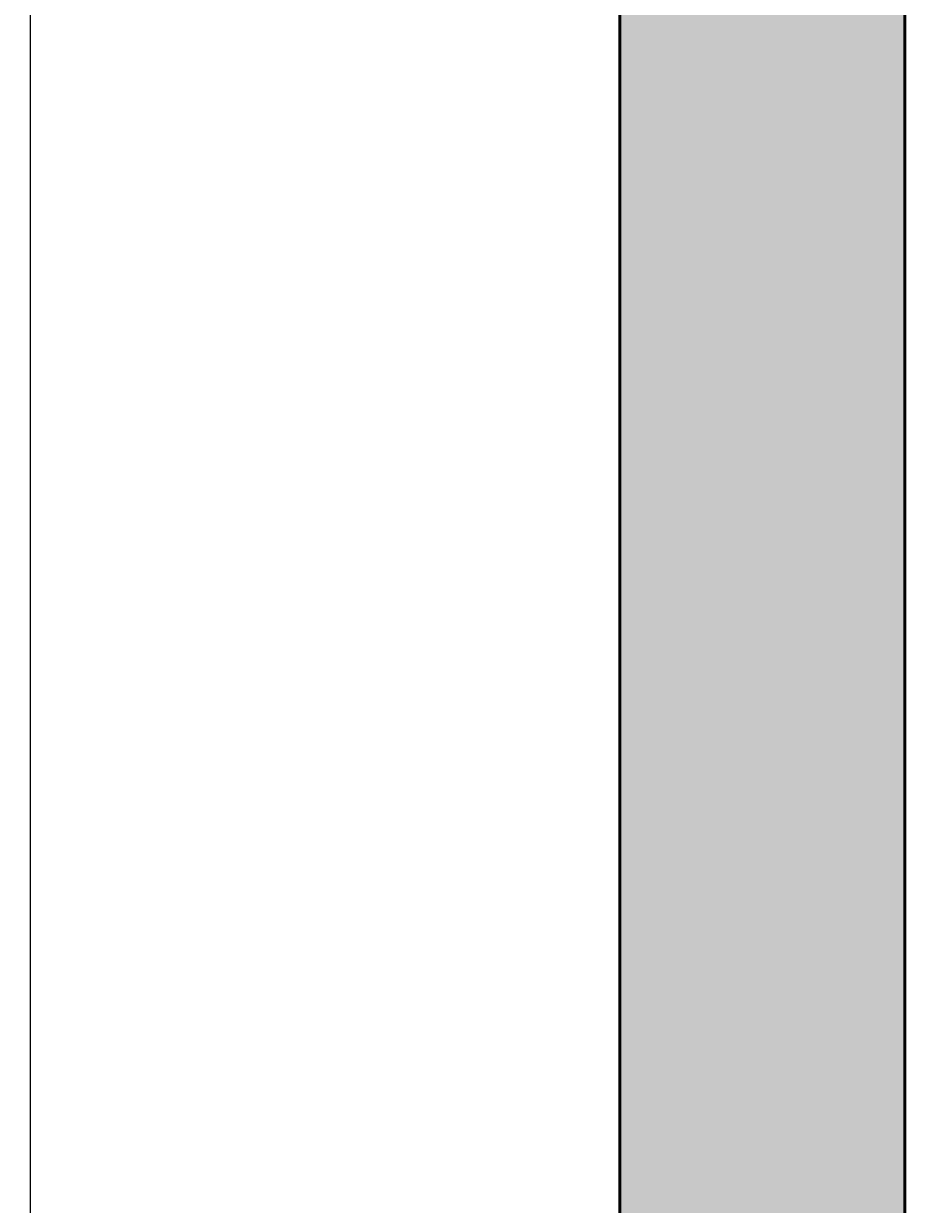
# Model space of a CAD drawing. Units: inches. Extents: x 2231 to 2461, y 2045 to 2455.
# Tile 71 of 95: x 2231 to 2260, y 2372 to 2409. Entities that reach past the tile are written whole.
import ezdxf

# ---------------------------------------------------------------- set-up
doc = ezdxf.new("R2010")
doc.units = ezdxf.units.IN
doc.layers.add('A-ANNO-DIMS', color=2, linetype='Continuous', lineweight=18)
doc.layers.add('A-WALL', color=7, linetype='Continuous', lineweight=50)
doc.layers.add('A-WALL-PATT', color=18, linetype='Continuous', lineweight=13, true_color=0x000000)
doc.styles.get("Standard").update_dxf_attribs({"font": 'arial.ttf'})
doc.dimstyles.get("Standard").update_dxf_attribs({"dimtxt": 0.18, "dimasz": 0.18, "dimexe": 0.18, "dimexo": 0.0625, "dimgap": 0.09, "dimtad": 0, "dimtih": 1, "dimtoh": 1, "dimdec": 4, "dimzin": 0, "dimdsep": 46, "dimtxsty": 'Standard', "dimcen": 0.09, "dimadec": 0, "dimazin": 0, "dimtfac": 1, "dimtdec": 4, "dimtofl": 0, "dimtmove": 0, "dimatfit": 3, "dimfxl": 1, "dimtolj": 1, "dimtzin": 0, "dimarcsym": 0})

# ---------------------------------------------------------------- blocks, each defined once
blk = doc.blocks.new('*D37')
at = {"layer": 'A-ANNO-DIMS', "color": 0, "lineweight": -2, "transparency": 16777216}
for p, q in [((2258.731, 2426.833), (2230.981, 2426.833)), ((2231.161, 2426.653), (2231.161, 2367.015)), ((2231.161, 2307.013), (2231.161, 2366.651)), ((2258.731, 2306.833), (2230.981, 2306.833))]:
    blk.add_line(p, q, dxfattribs=at)
at = {"layer": 'A-ANNO-DIMS', "color": 0, "transparency": 16777216}
for points in [[(2231.131, 2426.653), (2231.191, 2426.653), (2231.161, 2426.833)], [(2231.131, 2307.013), (2231.191, 2307.013), (2231.161, 2306.833)]]:
    blk.add_solid(points, dxfattribs=at)
at = {"layer": 'Defpoints', "color": 0, "transparency": 16777216}
for p in [(2231.161, 2426.833), (2258.794, 2426.833), (2258.794, 2306.833)]:
    blk.add_point(p, dxfattribs=at)
at = {"layer": 'A-ANNO-DIMS', "color": 0, "transparency": 16777216, "insert": (2231.161, 2366.833), "char_height": 0.18, "attachment_point": 5}
blk.add_mtext('\\A1;120', dxfattribs=at)
blk = doc.blocks.new('*D47')
at = {"layer": 'A-ANNO-DIMS', "color": 0, "lineweight": -2, "transparency": 16777216}
for p, q in [((2258.794, 2182.895), (2258.794, 2454.645)), ((2294.794, 2182.895), (2294.794, 2454.645)), ((2258.974, 2454.465), (2276.575, 2454.465)), ((2294.614, 2454.465), (2277.012, 2454.465))]:
    blk.add_line(p, q, dxfattribs=at)
at = {"layer": 'A-ANNO-DIMS', "color": 0, "transparency": 16777216}
for points in [[(2258.974, 2454.495), (2258.974, 2454.435), (2258.794, 2454.465)], [(2294.614, 2454.495), (2294.614, 2454.435), (2294.794, 2454.465)]]:
    blk.add_solid(points, dxfattribs=at)
at = {"layer": 'Defpoints', "color": 0, "transparency": 16777216}
for p in [(2294.794, 2454.465), (2258.794, 2182.833), (2294.794, 2182.833)]:
    blk.add_point(p, dxfattribs=at)
at = {"layer": 'A-ANNO-DIMS', "color": 0, "transparency": 16777216, "insert": (2276.794, 2454.465), "char_height": 0.18, "attachment_point": 5}
blk.add_mtext('\\A1;36', dxfattribs=at)

msp = doc.modelspace()

# ---------------------------------------------------------------- hatches: boundary and pattern name
at = {"layer": 'A-WALL-PATT'}
h = msp.add_hatch(color=256, dxfattribs=at)
h.dxf.hatch_style = 1
h.paths.add_polyline_path([(2441.7935, 2269.1535), (2432.7935, 2269.1535), (2432.7935, 2186.8328), (2396.7935, 2186.8328), (2396.7935, 2286.8328), (2394.7935, 2286.8328), (2394.7935, 2186.8328), (2334.7935, 2186.8328), (2334.7935, 2182.8328), (2432.7935, 2182.8328), (2432.7935, 2072.8328), (2416.6639, 2072.8328), (2416.6639, 2063.8328), (2441.7935, 2063.8328)])
h.paths.add_polyline_path([(2368.6639, 2072.8328), (2367.04, 2072.8328), (2330.7942, 2072.8328), (2330.7397, 2063.8328), (2368.6639, 2063.8328)])
h.paths.add_polyline_path([(2300.7392, 2068.3328), (2300.7392, 2072.8328), (2298.7935, 2072.8328), (2294.7935, 2072.8328), (2258.7935, 2072.8328), (2258.7935, 2120.8328), (2294.7935, 2120.8328), (2298.7935, 2120.8328), (2298.7935, 2128.8328), (2294.7935, 2128.8328), (2294.7935, 2124.8328), (2258.7935, 2124.8328), (2258.7935, 2182.8328), (2294.7935, 2182.8328), (2294.7935, 2174.8328), (2298.7935, 2174.8328), (2298.7935, 2182.8328), (2304.7935, 2182.8328), (2304.7935, 2186.8328), (2258.7935, 2186.8328), (2258.7935, 2221.999), (2249.7935, 2221.999), (2249.7935, 2063.8328), (2300.7392, 2063.8328)])
h.paths.add_polyline_path([(2391.9338, 2435.8328), (2333.82, 2435.8328), (2333.82, 2426.8328), (2368.7935, 2426.8328), (2368.7935, 2374.9508), (2368.7935, 2370.8328), (2372.3935, 2370.8328), (2372.7935, 2370.8328), (2372.7935, 2426.8328), (2391.9338, 2426.8328)])
h.paths.add_polyline_path([(2441.7935, 2435.8328), (2415.9338, 2435.8328), (2415.9338, 2426.8328), (2432.7935, 2426.8328), (2432.7935, 2334.8328), (2372.7935, 2334.8328), (2372.7935, 2346.8328), (2368.7935, 2346.8328), (2368.7935, 2306.8328), (2360.7935, 2306.8328), (2360.7935, 2302.8328), (2368.7935, 2302.8328), (2372.7935, 2302.8328), (2372.7935, 2330.8328), (2432.7935, 2330.8328), (2432.7935, 2317.1535), (2441.7935, 2317.1535)])
h.paths.add_polyline_path([(2285.82, 2435.8328), (2249.7935, 2435.8328), (2249.7935, 2269.999), (2258.7935, 2269.999), (2258.7935, 2302.8328), (2318.8168, 2302.8328), (2330.7935, 2302.8328), (2330.7935, 2306.8328), (2258.7935, 2306.8328), (2258.7935, 2426.8328), (2285.82, 2426.8328)])

# ---------------------------------------------------------------- linework, layer by layer
at = {"layer": 'A-WALL'}
msp.add_line((2258.7935, 2306.8328), (2258.7935, 2426.8328), dxfattribs=at)
msp.add_lwpolyline([(2300.7392, 2063.8328), (2249.7935, 2063.8328), (2249.7935, 2435.8328), (2441.7935, 2435.8328), (2441.7935, 2063.8328), (2330.7397, 2063.8328)], dxfattribs=at)

# ---------------------------------------------------------------- dimensions: what is measured, and where the dimension line sits
at = {"layer": 'A-ANNO-DIMS'}
dim = msp.add_linear_dim(base=(2294.7935, 2454.4653), p1=(2258.7935, 2182.8328), p2=(2294.7935, 2182.8328), dimstyle='Standard', override={"dimdec": 0, "dimlfac": 1, "dimrnd": 0, "dimzin": 0, "dimdsep": 46, "dimlunit": 2}, dxfattribs=at)
dim.commit()
dim.dimension.update_dxf_attribs({"geometry": '*D47', "text_midpoint": (2276.7935, 2454.4653)})
dim = msp.add_linear_dim(base=(2231.161, 2426.8328), p1=(2258.7935, 2306.8328), p2=(2258.7935, 2426.8328), angle=90, dimstyle='Standard', override={"dimdec": 0, "dimlfac": 1, "dimrnd": 0, "dimzin": 0, "dimdsep": 46, "dimlunit": 2}, dxfattribs=at)
dim.commit()
dim.dimension.update_dxf_attribs({"geometry": '*D37', "text_midpoint": (2231.161, 2366.8328)})

doc.saveas('drawing.dxf')
